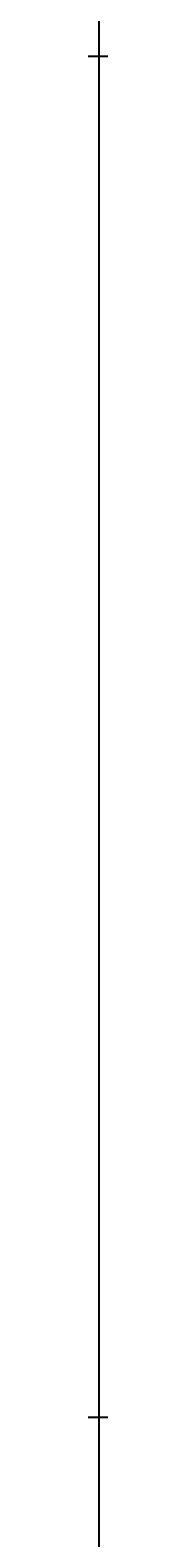
# Model space of a CAD drawing. Units: inches. Extents: x 35362 to 73946, y 43607 to 67532.
# Tile 25 of 134: x 48373 to 48373, y 46091 to 46564. Entities that reach past the tile are written whole.
import ezdxf

# ---------------------------------------------------------------- set-up
doc = ezdxf.new("R2010")
doc.units = ezdxf.units.IN
doc.header["$MEASUREMENT"] = 0
doc.layers.add('A-ANNO-DIMS', color=2, linetype='Continuous', lineweight=18)
doc.styles.get("Standard").update_dxf_attribs({"font": 'arial.ttf'})
doc.dimstyles.get("Standard").update_dxf_attribs({"dimtxt": 0.18, "dimasz": 0.18, "dimexe": 0.18, "dimexo": 0.0625, "dimgap": 0.09, "dimtad": 0, "dimtih": 1, "dimtoh": 1, "dimdec": 4, "dimzin": 0, "dimdsep": 46, "dimtxsty": 'Standard', "dimcen": 0.09, "dimadec": 0, "dimazin": 0, "dimtfac": 1, "dimtdec": 4, "dimtofl": 0, "dimtmove": 0, "dimatfit": 3, "dimfxl": 1, "dimtolj": 1, "dimtzin": 0, "dimarcsym": 0})

# ---------------------------------------------------------------- blocks, each defined once
blk = doc.blocks.new('*D5')
at = {"layer": 'A-ANNO-DIMS', "color": 0, "lineweight": -2, "transparency": 16777216}
for p, q in [((37121.95, 46919.32), (37121.95, 43606.68)), ((69871.5, 45449.83), (69871.5, 43606.68)), ((37122.13, 43606.86), (53496.29, 43606.86)), ((69871.32, 43606.86), (53497.15, 43606.86))]:
    blk.add_line(p, q, dxfattribs=at)
at = {"layer": 'A-ANNO-DIMS', "color": 0, "transparency": 16777216}
for points in [[(37122.13, 43606.89), (37122.13, 43606.83), (37121.95, 43606.86)], [(69871.32, 43606.89), (69871.32, 43606.83), (69871.5, 43606.86)]]:
    blk.add_solid(points, dxfattribs=at)
at = {"layer": 'Defpoints', "color": 0, "transparency": 16777216}
for p in [(37121.95, 46919.38), (69871.5, 45449.89), (69871.5, 43606.86)]:
    blk.add_point(p, dxfattribs=at)
at = {"layer": 'A-ANNO-DIMS', "color": 0, "transparency": 16777216, "insert": (53496.72, 43606.86), "char_height": 0.18, "attachment_point": 5}
blk.add_mtext('\\A1;32750', dxfattribs=at)
blk = doc.blocks.new('*D11')
at = {"layer": 'A-ANNO-DIMS', "color": 0, "lineweight": -2, "transparency": 16777216}
for p, q in [((47978.66, 56028.77), (47978.66, 43606.68)), ((53109.76, 56028.77), (53109.76, 43606.68)), ((47978.84, 43606.86), (50543.87, 43606.86)), ((53109.58, 43606.86), (50544.55, 43606.86))]:
    blk.add_line(p, q, dxfattribs=at)
at = {"layer": 'A-ANNO-DIMS', "color": 0, "transparency": 16777216}
for points in [[(47978.84, 43606.89), (47978.84, 43606.83), (47978.66, 43606.86)], [(53109.58, 43606.89), (53109.58, 43606.83), (53109.76, 43606.86)]]:
    blk.add_solid(points, dxfattribs=at)
at = {"layer": 'Defpoints', "color": 0, "transparency": 16777216}
for p in [(47978.66, 56028.84), (53109.76, 56028.84), (53109.76, 43606.86)]:
    blk.add_point(p, dxfattribs=at)
at = {"layer": 'A-ANNO-DIMS', "color": 0, "transparency": 16777216, "insert": (50544.21, 43606.86), "char_height": 0.18, "attachment_point": 5}
blk.add_mtext('\\A1;5131', dxfattribs=at)
blk = doc.blocks.new('*D27')
at = {"layer": 'A-ANNO-DIMS', "color": 0, "lineweight": -2, "transparency": 16777216}
for p, q in [((47978.66, 56028.77), (47978.66, 43606.68)), ((48373.49, 53428.96), (48373.49, 43606.68)), ((47978.84, 43606.86), (48175.68, 43606.86)), ((48373.31, 43606.86), (48176.47, 43606.86))]:
    blk.add_line(p, q, dxfattribs=at)
at = {"layer": 'A-ANNO-DIMS', "color": 0, "transparency": 16777216}
for points in [[(47978.84, 43606.89), (47978.84, 43606.83), (47978.66, 43606.86)], [(48373.31, 43606.89), (48373.31, 43606.83), (48373.49, 43606.86)]]:
    blk.add_solid(points, dxfattribs=at)
at = {"layer": 'Defpoints', "color": 0, "transparency": 16777216}
for p in [(47978.66, 56028.84), (48373.49, 53429.02), (48373.49, 43606.86)]:
    blk.add_point(p, dxfattribs=at)
at = {"layer": 'A-ANNO-DIMS', "color": 0, "transparency": 16777216, "insert": (48176.08, 43606.86), "char_height": 0.18, "attachment_point": 5}
blk.add_mtext('\\A1;394.8', dxfattribs=at)
blk = doc.blocks.new('*D67')
at = {"layer": 'A-ANNO-DIMS', "color": 0, "lineweight": -2, "transparency": 16777216}
for p, q in [((56873.54, 53351.53), (35361.77, 53351.53)), ((35361.95, 53351.35), (35361.95, 49400.89)), ((35361.95, 45450.07), (35361.95, 49400.53)), ((53793.58, 45449.89), (35361.77, 45449.89))]:
    blk.add_line(p, q, dxfattribs=at)
at = {"layer": 'A-ANNO-DIMS', "color": 0, "transparency": 16777216}
for points in [[(35361.92, 53351.35), (35361.98, 53351.35), (35361.95, 53351.53)], [(35361.92, 45450.07), (35361.98, 45450.07), (35361.95, 45449.89)]]:
    blk.add_solid(points, dxfattribs=at)
at = {"layer": 'Defpoints', "color": 0, "transparency": 16777216}
for p in [(35361.95, 53351.53), (56873.6, 53351.53), (53793.64, 45449.89)]:
    blk.add_point(p, dxfattribs=at)
at = {"layer": 'A-ANNO-DIMS', "color": 0, "transparency": 16777216, "insert": (35361.95, 49400.71), "char_height": 0.18, "attachment_point": 5}
blk.add_mtext('\\A1;7901.6', dxfattribs=at)
blk = doc.blocks.new('*D76')
at = {"layer": 'A-ANNO-DIMS', "color": 0, "lineweight": -2, "transparency": 16777216}
for p, q in [((54052.84, 46555.29), (35361.77, 46555.29)), ((35361.95, 46555.11), (35361.95, 46342.27)), ((35361.95, 46129.06), (35361.95, 46341.9)), ((53793.58, 46128.88), (35361.77, 46128.88))]:
    blk.add_line(p, q, dxfattribs=at)
at = {"layer": 'A-ANNO-DIMS', "color": 0, "transparency": 16777216}
for points in [[(35361.92, 46555.11), (35361.98, 46555.11), (35361.95, 46555.29)], [(35361.92, 46129.06), (35361.98, 46129.06), (35361.95, 46128.88)]]:
    blk.add_solid(points, dxfattribs=at)
at = {"layer": 'Defpoints', "color": 0, "transparency": 16777216}
for p in [(35361.95, 46555.29), (54052.9, 46555.29), (53793.64, 46128.88)]:
    blk.add_point(p, dxfattribs=at)
at = {"layer": 'A-ANNO-DIMS', "color": 0, "transparency": 16777216, "insert": (35361.95, 46342.09), "char_height": 0.18, "attachment_point": 5}
blk.add_mtext('\\A1;426.4', dxfattribs=at)
blk = doc.blocks.new('*D90')
at = {"layer": 'A-ANNO-DIMS', "color": 0, "lineweight": -2, "transparency": 16777216}
for p, q in [((53707.72, 47291.29), (35361.77, 47291.29)), ((35361.95, 47291.11), (35361.95, 46710.26)), ((35361.95, 46129.06), (35361.95, 46709.9)), ((53793.58, 46128.88), (35361.77, 46128.88))]:
    blk.add_line(p, q, dxfattribs=at)
at = {"layer": 'A-ANNO-DIMS', "color": 0, "transparency": 16777216}
for points in [[(35361.92, 47291.11), (35361.98, 47291.11), (35361.95, 47291.29)], [(35361.92, 46129.06), (35361.98, 46129.06), (35361.95, 46128.88)]]:
    blk.add_solid(points, dxfattribs=at)
at = {"layer": 'Defpoints', "color": 0, "transparency": 16777216}
for p in [(53707.78, 47291.29), (35361.95, 46128.88), (53793.64, 46128.88)]:
    blk.add_point(p, dxfattribs=at)
at = {"layer": 'A-ANNO-DIMS', "color": 0, "transparency": 16777216, "insert": (35361.95, 46710.08), "char_height": 0.18, "attachment_point": 5}
blk.add_mtext('\\A1;1162.4', dxfattribs=at)

msp = doc.modelspace()

# ---------------------------------------------------------------- dimensions: what is measured, and where the dimension line sits
at = {"layer": 'A-ANNO-DIMS'}
for base, p1, p2, override, picture, middle in [((53109.76, 43606.859), (47978.665, 56028.836), (53109.76, 56028.836), {"dimdec": 0, "dimlfac": 1, "dimrnd": 0, "dimzin": 0, "dimdsep": 46, "dimlunit": 2}, '*D11', (50544.212, 43606.859)), ((48373.492, 43606.859), (47978.665, 56028.836), (48373.492, 53429.019), {"dimdec": 1, "dimlfac": 1, "dimrnd": 0, "dimzin": 0, "dimdsep": 46, "dimlunit": 2}, '*D27', (48176.078, 43606.859)), ((69871.496, 43606.859), (37121.949, 46919.381), (69871.496, 45449.894), {"dimdec": 0, "dimlfac": 1, "dimrnd": 0, "dimzin": 0, "dimdsep": 46, "dimlunit": 2}, '*D5', (53496.723, 43606.859))]:
    dim = msp.add_linear_dim(base=base, p1=p1, p2=p2, dimstyle='Standard', override=override, dxfattribs=at)
    dim.commit()
    dim.dimension.update_dxf_attribs({"geometry": picture, "text_midpoint": middle})
for base, p1, p2, picture, middle in [((35361.949, 53351.529), (53793.638, 45449.894), (56873.602, 53351.529), '*D67', (35361.949, 49400.712)), ((35361.949, 46128.878), (53707.781, 47291.285), (53793.638, 46128.878), '*D90', (35361.949, 46710.081)), ((35361.949, 46555.293), (53793.638, 46128.878), (54052.899, 46555.293), '*D76', (35361.949, 46342.086))]:
    dim = msp.add_linear_dim(base=base, p1=p1, p2=p2, angle=90, dimstyle='Standard', override={"dimdec": 1, "dimlfac": 1, "dimrnd": 0, "dimzin": 0, "dimdsep": 46, "dimlunit": 2}, dxfattribs=at)
    dim.commit()
    dim.dimension.update_dxf_attribs({"geometry": picture, "text_midpoint": middle})

doc.saveas('drawing.dxf')
